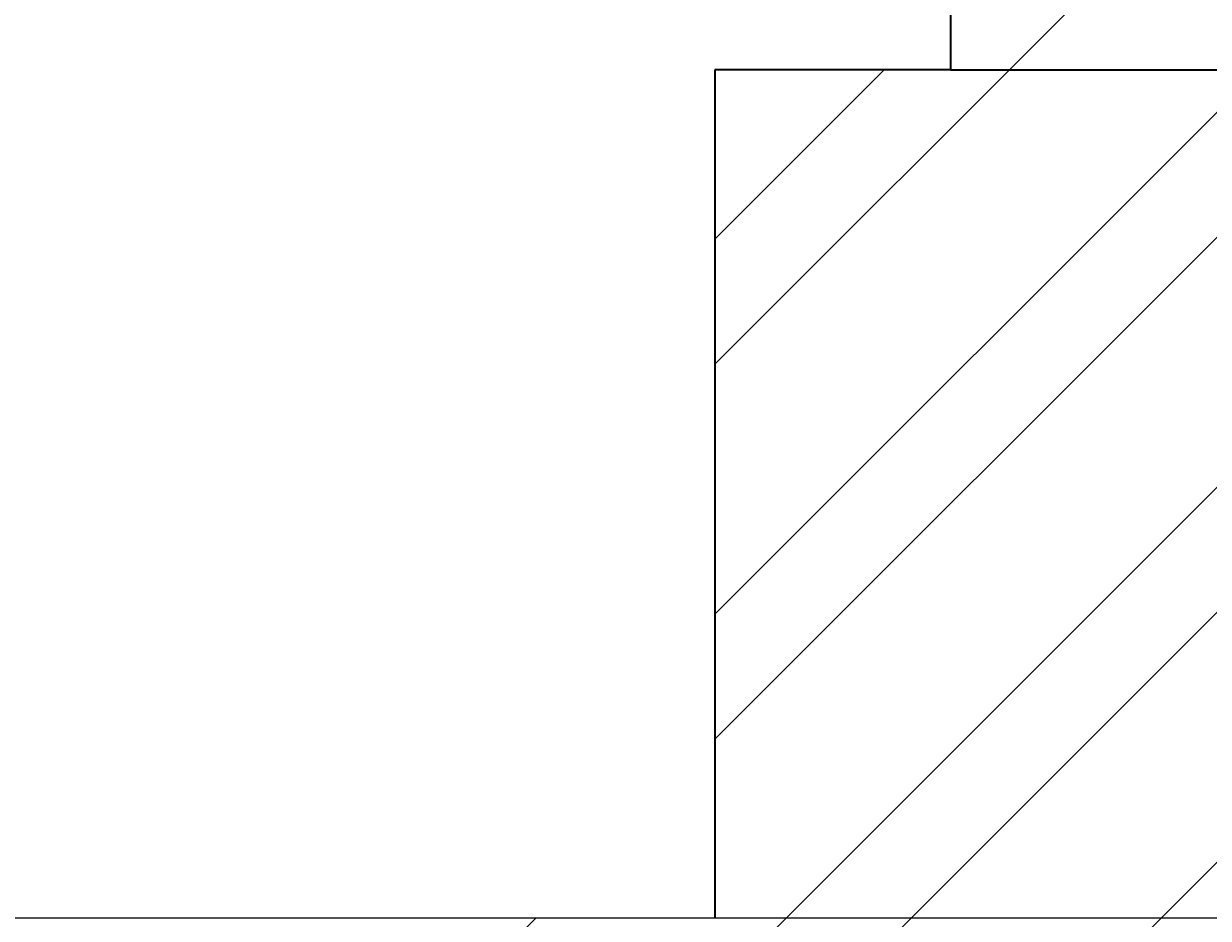
# Model space of a CAD drawing. Units: inches. Extents: x -301 to 715, y -607 to 364.
# Tile 7 of 141: x -66 to -41, y -511 to -492. Entities that reach past the tile are written whole.
import ezdxf

# ---------------------------------------------------------------- set-up
doc = ezdxf.new("R2010")
doc.units = ezdxf.units.IN
doc.header["$MEASUREMENT"] = 0
for name, color, linetype, lineweight in [('A-ANNO-DIMS', 2, 'Continuous', 18), ('A-SECT-PATT', 8, 'Continuous', 13), ('S-FNDN', 2, 'Continuous', 35)]:
    doc.layers.add(name, color=color, linetype=linetype, lineweight=lineweight)
doc.styles.get("Standard").update_dxf_attribs({"font": 'arial.ttf'})
doc.dimstyles.get("Standard").update_dxf_attribs({"dimtxt": 0.18, "dimasz": 0.18, "dimexe": 0.18, "dimexo": 0.0625, "dimgap": 0.09, "dimtad": 0, "dimtih": 1, "dimtoh": 1, "dimdec": 1, "dimzin": 0, "dimdsep": 46, "dimlunit": 4, "dimtxsty": 'Standard', "dimcen": 0.09, "dimclrd": 3, "dimclre": 4, "dimclrt": 6, "dimadec": 0, "dimazin": 0, "dimtfac": 1, "dimtdec": 1, "dimtofl": 0, "dimtmove": 0, "dimatfit": 3, "dimfxl": 1, "dimtfill": 2, "dimtfillclr": 51, "dimtolj": 1, "dimtzin": 0, "dimarcsym": 0})

# ---------------------------------------------------------------- blocks, each defined once
blk = doc.blocks.new('*D179')
at = {"layer": 'A-ANNO-DIMS', "color": 4, "lineweight": -2, "transparency": 16777216}
for p, q in [((-87.981, -433.54), (-87.981, -573.809)), ((-35.282, -463.54), (-35.282, -573.809))]:
    blk.add_line(p, q, dxfattribs=at)
at = {"layer": 'A-ANNO-DIMS', "color": 3, "lineweight": -2, "transparency": 16777216}
for p, q in [((-87.801, -573.629), (-62.174, -573.629)), ((-35.462, -573.629), (-61.089, -573.629))]:
    blk.add_line(p, q, dxfattribs=at)
at = {"layer": 'A-ANNO-DIMS', "color": 3, "transparency": 16777216}
for points in [[(-87.801, -573.599), (-87.801, -573.659), (-87.981, -573.629)], [(-35.462, -573.599), (-35.462, -573.659), (-35.282, -573.629)]]:
    blk.add_solid(points, dxfattribs=at)
at = {"layer": 'Defpoints', "color": 0, "transparency": 16777216}
for p in [(-87.981, -433.477), (-35.282, -463.477), (-35.282, -573.629)]:
    blk.add_point(p, dxfattribs=at)
at = {"layer": 'A-ANNO-DIMS', "color": 6, "transparency": 16777216, "insert": (-61.631, -573.629), "char_height": 0.18, "attachment_point": 5, "bg_fill": 1, "box_fill_scale": 1.25, "bg_fill_color": 51, "bg_fill_transparency": 0}
blk.add_mtext('\\A1;4\'-4 1/2"', dxfattribs=at)
blk = doc.blocks.new('*D190')
at = {"layer": 'A-ANNO-DIMS', "color": 4, "lineweight": -2, "transparency": 16777216}
for p, q in [((129.193, -481.477), (-266.112, -481.477)), ((124.193, -511.477), (-266.112, -511.477))]:
    blk.add_line(p, q, dxfattribs=at)
at = {"layer": 'A-ANNO-DIMS', "color": 3, "lineweight": -2, "transparency": 16777216}
for p, q in [((-265.932, -481.657), (-265.932, -496.296)), ((-265.932, -511.297), (-265.932, -496.659))]:
    blk.add_line(p, q, dxfattribs=at)
at = {"layer": 'A-ANNO-DIMS', "color": 3, "transparency": 16777216}
for points in [[(-265.962, -481.657), (-265.902, -481.657), (-265.932, -481.477)], [(-265.962, -511.297), (-265.902, -511.297), (-265.932, -511.477)]]:
    blk.add_solid(points, dxfattribs=at)
at = {"layer": 'Defpoints', "color": 0, "transparency": 16777216}
for p in [(129.255, -481.477), (-265.932, -511.477), (124.255, -511.477)]:
    blk.add_point(p, dxfattribs=at)
at = {"layer": 'A-ANNO-DIMS', "color": 6, "transparency": 16777216, "insert": (-265.932, -496.477), "char_height": 0.18, "attachment_point": 5, "bg_fill": 1, "box_fill_scale": 1.25, "bg_fill_color": 51, "bg_fill_transparency": 0}
blk.add_mtext('\\A1;2\'-6"', dxfattribs=at)
blk = doc.blocks.new('*D191')
at = {"layer": 'A-ANNO-DIMS', "color": 4, "lineweight": -2, "transparency": 16777216}
for p, q in [((129.193, -481.477), (-266.112, -481.477)), ((114.193, -540.477), (-266.112, -540.477))]:
    blk.add_line(p, q, dxfattribs=at)
at = {"layer": 'A-ANNO-DIMS', "color": 3, "lineweight": -2, "transparency": 16777216}
for p, q in [((-265.932, -481.657), (-265.932, -510.797)), ((-265.932, -540.297), (-265.932, -511.158))]:
    blk.add_line(p, q, dxfattribs=at)
at = {"layer": 'A-ANNO-DIMS', "color": 3, "transparency": 16777216}
for points in [[(-265.962, -481.657), (-265.902, -481.657), (-265.932, -481.477)], [(-265.962, -540.297), (-265.902, -540.297), (-265.932, -540.477)]]:
    blk.add_solid(points, dxfattribs=at)
at = {"layer": 'Defpoints', "color": 0, "transparency": 16777216}
for p in [(129.255, -481.477), (-265.932, -540.477), (114.255, -540.477)]:
    blk.add_point(p, dxfattribs=at)
at = {"layer": 'A-ANNO-DIMS', "color": 6, "transparency": 16777216, "insert": (-265.932, -510.977), "char_height": 0.18, "attachment_point": 5, "bg_fill": 1, "box_fill_scale": 1.25, "bg_fill_color": 51, "bg_fill_transparency": 0}
blk.add_mtext('\\A1;4\'-11"', dxfattribs=at)

msp = doc.modelspace()

# ---------------------------------------------------------------- hatches: boundary and pattern name
at = {"layer": 'A-SECT-PATT'}
h = msp.add_hatch(dxfattribs=at)
h.set_pattern_fill('ANSI32', color=256, scale=15)
h.set_pattern_definition([(45, (10.321, 33.8764), (-3.977476, 3.977476), []), (45, (12.973, 33.8764), (-3.977476, 3.977476), [])])
h.paths.add_polyline_path([(-185.282, -324.477), (-199.282, -324.477), (-199.282, -329.477), (-194.282, -329.477), (-194.282, -353.477), (-185.282, -353.477)])
h.paths.add_polyline_path([(-185.282, -361.477), (-193.904, -361.477), (-193.982, -377.537), (-185.282, -377.537)])
h.paths.add_polyline_path([(143.218, -329.477), (148.218, -329.477), (148.218, -324.477), (134.255, -324.477), (134.255, -353.477), (143.218, -353.477)])
h.paths.add_polyline_path([(143.218, -361.477), (134.255, -361.477), (134.255, -377.477), (143.218, -377.477)])
h.paths.add_polyline_path([(-185.282, -439.477), (-194.282, -439.477), (-194.282, -463.477), (-185.282, -463.477)])
h.paths.add_polyline_path([(-185.282, -471.477), (-194.282, -471.477), (-194.282, -481.477), (-185.282, -481.477)])
h.paths.add_polyline_path([(-185.282, -463.477), (-194.282, -463.477), (-194.282, -466.477), (-185.282, -466.477)])
h.paths.add_polyline_path([(-185.282, -466.477), (-194.282, -466.477), (-194.282, -471.477), (-185.282, -471.477)])
h.paths.add_polyline_path([(-180.282, -481.477), (-185.282, -481.477), (-194.282, -481.477), (-199.282, -481.477), (-199.282, -493.477), (-180.282, -493.477)])
h.paths.add_polyline_path([(-175.282, -493.477), (-180.282, -493.477), (-199.282, -493.477), (-204.282, -493.477), (-204.282, -511.477), (-175.282, -511.477)])
h.paths.add_polyline_path([(-170.282, -511.477), (-175.282, -511.477), (-204.282, -511.477), (-209.282, -511.477), (-209.282, -535.477), (-170.282, -535.477)])
h.paths.add_polyline_path([(-35.282, -463.477), (-41.282, -463.477), (-41.282, -466.477), (-35.282, -466.477)])
h.paths.add_polyline_path([(-35.282, -466.477), (-41.282, -466.477), (-41.282, -471.477), (-35.282, -471.477)])
h.paths.add_polyline_path([(-35.282, -471.477), (-41.282, -471.477), (-41.282, -481.477), (-35.282, -481.477)])
h.paths.add_polyline_path([(-30.282, -481.477), (-46.282, -481.477), (-46.282, -493.477), (-30.282, -493.477)])
h.paths.add_polyline_path([(-25.282, -493.477), (-30.282, -493.477), (-46.282, -493.477), (-51.282, -493.477), (-51.282, -511.477), (-25.282, -511.477)])
h.paths.add_polyline_path([(-20.282, -511.477), (-25.282, -511.477), (-51.282, -511.477), (-56.282, -511.477), (-56.282, -535.477), (-20.282, -535.477)])
h.paths.add_polyline_path([(143.218, -463.477), (134.255, -463.477), (134.255, -466.477), (143.218, -466.477)])
h.paths.add_polyline_path([(143.218, -466.477), (134.255, -466.477), (134.255, -471.477), (143.218, -471.477)])
h.paths.add_polyline_path([(143.218, -471.477), (134.255, -471.477), (134.255, -481.477), (143.218, -481.477)])
h.paths.add_polyline_path([(148.255, -481.477), (143.255, -481.477), (134.255, -481.477), (129.255, -481.477), (129.255, -493.477), (148.255, -493.477)])
h.paths.add_polyline_path([(153.255, -493.477), (148.255, -493.477), (129.255, -493.477), (124.255, -493.477), (124.255, -511.477), (153.255, -511.477)])
h.paths.add_polyline_path([(158.255, -511.477), (153.255, -511.477), (124.255, -511.477), (119.255, -511.477), (119.255, -535.477), (158.255, -535.477)])

# ---------------------------------------------------------------- linework, layer by layer
at = {"layer": 'S-FNDN'}
for p, q in [((-46.282, -481.477), (-46.282, -493.477)), ((-46.282, -493.477), (-51.282, -493.477)), ((-51.282, -493.477), (-51.282, -511.477)), ((-46.282, -493.477), (-30.282, -493.477))]:
    msp.add_line(p, q, dxfattribs=at)

# ---------------------------------------------------------------- dimensions: what is measured, and where the dimension line sits
at = {"layer": 'A-ANNO-DIMS'}
dim = msp.add_linear_dim(base=(-35.282, -573.629), p1=(-87.981, -433.477), p2=(-35.282, -463.477), dimstyle='Standard', override={"dimdec": 1, "dimlfac": 1, "dimrnd": 0, "dimzin": 1, "dimdsep": 46, "dimlunit": 4, "dimfrac": 2}, dxfattribs=at)
dim.commit()
dim.dimension.update_dxf_attribs({"geometry": '*D179', "text_midpoint": (-61.631, -573.629)})
for base, p2, picture, middle in [((-265.932, -540.477), (114.255, -540.477), '*D191', (-265.932, -510.977)), ((-265.932, -511.477), (124.255, -511.477), '*D190', (-265.932, -496.477))]:
    dim = msp.add_linear_dim(base=base, p1=(129.255, -481.477), p2=p2, angle=90, dimstyle='Standard', override={"dimdec": 1, "dimlfac": 1, "dimrnd": 0, "dimzin": 1, "dimdsep": 46, "dimlunit": 4, "dimfrac": 2}, dxfattribs=at)
    dim.commit()
    dim.dimension.update_dxf_attribs({"geometry": picture, "text_midpoint": middle})

doc.saveas('drawing.dxf')
